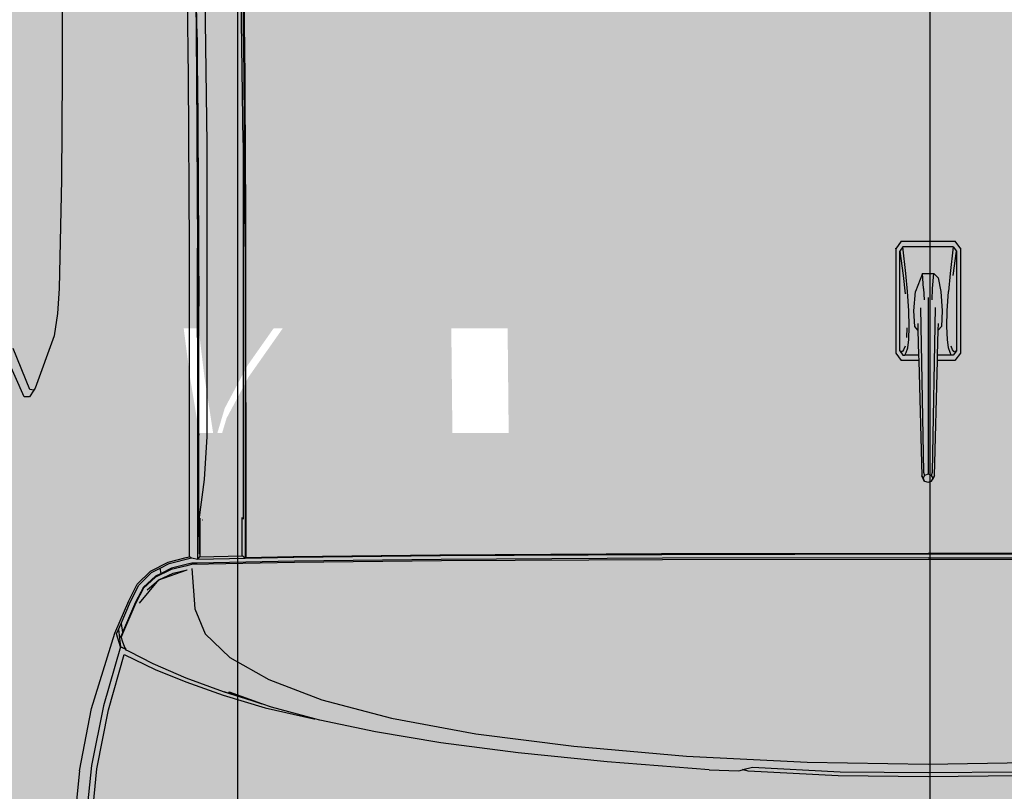
# Model space of a CAD drawing. Units: inches. Extents: x 1884 to 2398, y 474 to 1488.
# Tile 6 of 39: x 2203 to 2232, y 597 to 620. Entities that reach past the tile are written whole.
import ezdxf

# ---------------------------------------------------------------- set-up
doc = ezdxf.new("R2010")
doc.units = ezdxf.units.IN
doc.header["$MEASUREMENT"] = 0
doc.layers.get('0').update_dxf_attribs({"color": 250})
doc.layers.add('A-ANNO-DIMS', color=2, linetype='Continuous', lineweight=18)
doc.layers.add('C-VEHI', color=8, linetype='Continuous', lineweight=18)
doc.layers.add('Edges', color=250, linetype='Continuous')
doc.layers.add('L-PVMT-PATT', color=9, linetype='Continuous', lineweight=13, true_color=0xc7c8ca)
doc.styles.get("Standard").update_dxf_attribs({"font": 'arial.ttf'})
doc.dimstyles.get("Standard").update_dxf_attribs({"dimtxt": 7, "dimasz": 0.18, "dimexe": 0.18, "dimexo": 0.0625, "dimgap": 0.09, "dimtad": 0, "dimtih": 1, "dimtoh": 1, "dimzin": 0, "dimdsep": 46, "dimlunit": 3, "dimtxsty": 'Standard', "dimcen": 0.09, "dimadec": 0, "dimazin": 0, "dimtfac": 1, "dimtofl": 0, "dimtmove": 0, "dimatfit": 3, "dimfxl": 1, "dimtolj": 1, "dimtzin": 0, "dimarcsym": 0})

# ---------------------------------------------------------------- blocks, each defined once
blk = doc.blocks.new('Nissan Qashqai pl')
at = {"layer": 'Edges'}
for p, q in [((11.05474, 11.92208), (11.05507, 12.12031)), ((11.05537, 11.92208), (11.05571, 12.1202)), ((11.0586, 12.11975), (11.05827, 11.92208)), ((11.05972, 12.11965), (11.05938, 11.92208)), ((11.21164, 11.92208), (11.21014, 12.01197)), ((11.22044, 11.98904), (11.22108, 11.92208)), ((11.21801, 11.92208), (11.21745, 11.98742)), ((10.8228, 11.94208), (10.82834, 11.94608)), ((10.82794, 11.94608), (10.82834, 11.94608)), ((10.82834, 11.94608), (10.90603, 11.94608)), ((10.90603, 11.94608), (10.91157, 11.94208)), ((10.8228, 11.94208), (10.82239, 11.94208)), ((10.8228, 11.90208), (10.8228, 11.94208)), ((10.82696, 11.94083), (10.83007, 11.94308)), ((10.82696, 11.94083), (10.82696, 11.90333)), ((10.82696, 11.94083), (10.84666, 11.93861)), ((10.84833, 11.9406), (10.83007, 11.94308)), ((10.83007, 11.94308), (10.9043, 11.94308)), ((10.84666, 11.93861), (10.86027, 11.93735)), ((10.8746, 11.93634), (10.86027, 11.93735)), ((10.90215, 11.93722), (10.89593, 11.93645)), ((10.90348, 11.94026), (10.90076, 11.93914)), ((10.90565, 11.93837), (10.90215, 11.93722)), ((10.90503, 11.94137), (10.90348, 11.94026)), ((10.9043, 11.94308), (10.90741, 11.94083)), ((10.9043, 11.94308), (10.90503, 11.94137)), ((10.90744, 11.9393), (10.90565, 11.93837)), ((10.90741, 11.94083), (10.90744, 11.9393)), ((10.90744, 11.9393), (10.90744, 11.92915)), ((10.91157, 11.94208), (10.91157, 11.92904)), ((10.85007, 11.92947), (10.86027, 11.93157)), ((10.86027, 11.93157), (10.8746, 11.93265)), ((10.88611, 11.93611), (10.8746, 11.93634)), ((10.8746, 11.93265), (10.88611, 11.93193)), ((10.889, 11.92962), (10.88395, 11.92975)), ((10.89593, 11.93645), (10.88611, 11.93611)), ((10.88611, 11.93193), (10.889, 11.92962)), ((10.84666, 11.92634), (10.85007, 11.92947)), ((10.84666, 11.91782), (10.84666, 11.92634)), ((10.85787, 11.92547), (10.84666, 11.92634)), ((10.86624, 11.92503), (10.85787, 11.92547)), ((10.99456, 11.92544), (10.87195, 11.92764)), ((10.90744, 11.92915), (10.889, 11.92962)), ((10.91157, 11.92904), (10.90744, 11.92915)), ((10.99731, 11.92683), (10.91157, 11.92904)), ((10.99691, 11.92468), (10.99456, 11.92544)), ((10.99691, 11.92468), (10.99603, 11.92208)), ((10.99903, 11.92575), (10.99691, 11.92468)), ((10.99731, 11.92683), (11.00007, 11.92544)), ((10.99903, 11.92575), (10.99731, 11.92683)), ((11.00116, 11.92468), (10.99903, 11.92575)), ((11.00116, 11.92468), (11.00007, 11.92544)), ((11.00204, 11.92208), (11.00116, 11.92468)), ((10.85787, 11.91869), (10.84666, 11.91782)), ((10.84666, 11.91782), (10.86027, 11.91259)), ((10.85787, 11.91869), (10.86624, 11.91913)), ((10.86474, 11.92208), (10.99603, 11.92208)), ((10.87225, 11.91653), (10.99456, 11.91872)), ((10.90744, 11.91502), (10.91157, 11.91512)), ((10.91157, 11.91512), (10.99731, 11.91733)), ((10.91157, 11.91512), (10.91157, 11.90208)), ((10.99456, 11.91872), (10.99691, 11.91949)), ((10.99603, 11.92208), (10.99691, 11.91949)), ((10.99691, 11.91949), (10.99903, 11.91841)), ((11.00007, 11.91872), (10.99731, 11.91733)), ((10.99731, 11.91733), (10.99903, 11.91841)), ((10.99903, 11.91841), (10.99963, 11.91871)), ((10.99963, 11.91871), (11.00116, 11.91949)), ((11.00007, 11.91872), (10.99963, 11.91871)), ((11.00116, 11.91949), (11.00007, 11.91872)), ((11.00116, 11.91949), (11.00204, 11.92208)), ((11.05507, 11.72385), (11.05474, 11.92208)), ((11.05571, 11.72396), (11.05537, 11.92208)), ((11.05827, 11.92208), (11.0586, 11.72441)), ((11.05938, 11.92208), (11.05972, 11.72451)), ((11.21014, 11.8322), (11.21164, 11.92208)), ((11.21745, 11.85674), (11.21801, 11.92208)), ((11.22108, 11.92208), (11.22044, 11.85512)), ((10.8746, 11.91151), (10.86027, 11.91259)), ((10.8746, 11.90782), (10.86027, 11.90681)), ((10.88611, 11.91223), (10.8746, 11.91151)), ((10.88611, 11.90805), (10.8746, 11.90782)), ((10.88395, 11.91441), (10.889, 11.91454)), ((10.889, 11.91454), (10.88611, 11.91223)), ((10.89593, 11.90771), (10.88611, 11.90805)), ((10.889, 11.91454), (10.90744, 11.91502)), ((10.90744, 11.91502), (10.90744, 11.90486)), ((10.82239, 11.90208), (10.8228, 11.90208)), ((10.8228, 11.90208), (10.82834, 11.89808)), ((10.84666, 11.90555), (10.82696, 11.90333)), ((10.82696, 11.90333), (10.83007, 11.90108)), ((10.83007, 11.90108), (10.84833, 11.90356)), ((10.9043, 11.90108), (10.83007, 11.90108)), ((10.86027, 11.90681), (10.84666, 11.90555)), ((10.84833, 11.90356), (10.86193, 11.905)), ((10.88709, 11.90634), (10.89442, 11.90601)), ((10.90215, 11.90694), (10.89593, 11.90771)), ((10.90076, 11.90502), (10.90348, 11.9039)), ((10.90565, 11.90579), (10.90215, 11.90694)), ((10.90348, 11.9039), (10.90503, 11.90279)), ((10.9043, 11.90108), (10.90741, 11.90333)), ((10.90503, 11.90279), (10.9043, 11.90108)), ((10.90744, 11.90486), (10.90565, 11.90579)), ((10.90603, 11.89808), (10.91157, 11.90208)), ((10.90741, 11.90333), (10.90744, 11.90486)), ((10.90741, 11.90333), (10.90741, 11.90484)), ((10.82834, 11.89808), (10.82794, 11.89808)), ((10.82834, 11.89808), (10.90603, 11.89808)), ((11.2139, 11.7914), (11.21745, 11.85674)), ((11.22044, 11.85512), (11.21682, 11.78816)), ((11.20565, 11.74231), (11.21014, 11.8322)), ((11.21579, 11.78424), (11.2139, 11.7914)), ((11.21682, 11.78816), (11.21579, 11.78424)), ((11.21585, 11.78401), (11.21579, 11.78424)), ((11.21682, 11.78816), (11.21585, 11.78401)), ((11.21658, 11.78121), (11.21585, 11.78401)), ((11.21586, 11.75915), (11.21658, 11.78121)), ((11.21586, 11.75915), (11.20997, 11.68347)), ((11.19842, 11.65867), (11.20565, 11.74231)), ((11.05596, 11.55904), (11.05507, 11.72385)), ((11.0566, 11.5593), (11.05571, 11.72396)), ((11.0586, 11.72441), (11.05947, 11.55994)), ((11.05972, 11.72451), (11.06059, 11.56009)), ((11.20997, 11.68347), (11.2033, 11.61723)), ((11.18907, 11.58559), (11.19842, 11.65867)), ((11.2033, 11.61723), (11.19582, 11.55976)), ((11.17758, 11.52307), (11.18907, 11.58559)), ((11.05722, 11.44991), (11.05596, 11.55904)), ((11.05785, 11.45038), (11.0566, 11.5593)), ((11.05947, 11.55994), (11.06074, 11.45082)), ((11.06059, 11.56009), (11.06182, 11.4509)), ((11.19582, 11.55976), (11.18773, 11.51111)), ((11.16395, 11.47112), (11.17758, 11.52307)), ((11.18773, 11.51111), (11.17906, 11.46956)), ((11.14869, 11.43161), (11.16395, 11.47112)), ((11.17906, 11.46956), (11.17808, 11.46592)), ((11.17808, 11.46592), (11.1694, 11.43374)), ((11.1699, 11.42889), (11.17797, 11.4652)), ((11.17797, 11.4652), (11.17808, 11.46592)), ((11.05789, 11.4146), (11.05722, 11.44991)), ((11.05854, 11.41419), (11.05785, 11.45038)), ((11.06074, 11.45082), (11.06214, 11.37845)), ((11.06182, 11.4509), (11.06324, 11.37414)), ((11.1694, 11.43374), (11.1668, 11.42651)), ((11.1323, 11.40268), (11.14869, 11.43161)), ((11.1668, 11.42651), (11.1582, 11.40259)), ((11.16047, 11.39766), (11.1699, 11.42889)), ((11.16426, 11.41918), (11.1668, 11.42651)), ((11.15764, 11.39828), (11.16426, 11.41918)), ((11.15766, 11.39771), (11.16426, 11.41918)), ((11.16426, 11.41918), (11.15826, 11.40186)), ((10.69961, 11.41337), (10.55607, 11.41187)), ((10.5563, 11.41232), (10.69989, 11.41381)), ((10.7493, 11.41253), (10.62233, 11.41086)), ((10.77221, 11.41378), (10.69961, 11.41337)), ((10.69989, 11.41381), (10.77221, 11.4142)), ((10.7493, 11.41253), (11.02943, 11.41262)), ((10.77221, 11.4142), (10.78885, 11.41429)), ((10.77221, 11.4142), (10.77221, 11.41378)), ((10.78885, 11.41387), (10.77221, 11.41378)), ((10.78885, 11.41429), (10.79225, 11.41431)), ((10.78885, 11.41387), (10.78885, 11.41429)), ((10.79225, 11.41389), (10.78885, 11.41387)), ((10.79225, 11.41431), (10.79328, 11.41432)), ((10.79225, 11.41389), (10.79225, 11.41431)), ((10.79328, 11.4139), (10.79225, 11.41389)), ((10.79328, 11.41432), (10.82704, 11.4145)), ((10.79328, 11.4139), (10.79328, 11.41432)), ((10.82673, 11.41408), (10.79328, 11.4139)), ((10.82673, 11.41408), (11.05854, 11.41419)), ((10.82704, 11.4145), (11.05789, 11.4146)), ((11.02945, 11.41183), (11.02814, 11.41183)), ((11.02944, 11.41252), (11.02943, 11.41262)), ((11.05683, 11.41184), (11.02945, 11.41183)), ((11.02945, 11.41162), (11.02945, 11.41183)), ((11.05854, 11.41419), (11.05683, 11.41184)), ((11.05743, 11.38044), (11.05683, 11.41184)), ((11.05854, 11.41419), (11.05789, 11.4146)), ((11.05921, 11.37886), (11.05854, 11.41419)), ((11.11477, 11.38434), (11.1323, 11.40268)), ((11.14751, 11.37001), (11.15766, 11.39771)), ((11.15051, 11.36998), (11.16047, 11.39766)), ((10.62366, 11.38388), (10.75022, 11.38554)), ((10.75022, 11.38554), (10.96805, 11.38566)), ((10.96805, 11.38566), (10.99996, 11.38365)), ((10.99996, 11.38365), (11.03007, 11.37965)), ((11.03002, 11.38217), (11.03001, 11.38239)), ((11.03005, 11.38043), (11.05544, 11.38044)), ((11.05544, 11.38044), (11.03005, 11.38025)), ((11.05544, 11.38044), (11.05743, 11.38044)), ((11.05921, 11.37886), (11.05743, 11.38044)), ((11.09618, 11.37663), (11.11477, 11.38434)), ((10.55662, 11.37645), (10.69998, 11.37799)), ((10.6649, 11.37825), (10.55757, 11.37665)), ((10.6649, 11.37825), (10.58658, 11.37719)), ((10.69078, 11.37855), (10.6649, 11.37825)), ((10.6649, 11.37825), (10.67717, 11.37844)), ((10.69658, 11.37873), (10.67717, 11.37844)), ((10.67717, 11.37844), (10.69078, 11.37855)), ((10.69913, 11.37864), (10.69078, 11.37855)), ((10.71439, 11.37882), (10.69658, 11.37873)), ((10.69986, 11.37862), (10.69913, 11.37864)), ((10.69986, 11.37862), (10.78083, 11.37927)), ((10.71439, 11.37882), (10.69986, 11.37862)), ((10.69998, 11.37799), (10.82786, 11.37874)), ((10.72388, 11.37887), (10.71439, 11.37882)), ((10.72479, 11.37891), (10.72388, 11.37887)), ((10.78083, 11.37927), (10.72479, 11.37891)), ((10.78083, 11.37927), (10.8711, 11.37956)), ((10.94306, 11.3796), (10.82786, 11.37874)), ((10.82786, 11.37874), (11.05524, 11.37886)), ((10.96142, 11.37881), (10.82786, 11.37874)), ((10.89604, 11.37957), (10.8711, 11.37956)), ((10.90974, 11.3796), (10.89604, 11.37957)), ((10.94306, 11.3796), (10.90974, 11.3796)), ((10.94785, 11.37963), (10.94306, 11.3796)), ((10.9491, 11.37964), (10.94785, 11.37963)), ((10.96679, 11.37961), (10.9491, 11.37964)), ((10.96142, 11.37881), (10.96679, 11.37961)), ((10.97113, 11.37881), (10.96142, 11.37881)), ((10.96679, 11.37961), (10.96696, 11.37964)), ((10.97653, 11.37962), (10.96696, 11.37964)), ((10.97653, 11.37962), (10.97113, 11.37881)), ((10.97664, 11.37882), (10.97113, 11.37881)), ((10.98248, 11.37964), (10.97653, 11.37962)), ((10.97653, 11.37962), (10.97664, 11.37882)), ((11.05921, 11.37886), (10.97664, 11.37882)), ((11.03007, 11.37965), (10.98248, 11.37964)), ((11.02869, 11.38043), (11.03005, 11.38043)), ((11.03005, 11.38025), (11.02923, 11.38024)), ((11.03005, 11.38025), (11.03005, 11.38043)), ((11.03007, 11.37965), (11.03005, 11.38025)), ((11.05822, 11.37418), (11.05754, 11.37277)), ((11.05822, 11.37418), (11.05921, 11.37886)), ((11.06236, 11.3576), (11.05822, 11.37418)), ((11.06214, 11.37845), (11.06222, 11.37449)), ((11.06222, 11.37449), (11.06303, 11.37135)), ((11.06324, 11.37414), (11.06408, 11.37085)), ((11.06624, 11.37435), (11.09618, 11.37663)), ((10.7004, 11.37196), (10.55723, 11.37045)), ((10.82794, 11.37265), (10.7004, 11.37196)), ((11.05437, 11.37279), (10.82794, 11.37265)), ((11.05754, 11.37277), (11.05437, 11.37279)), ((11.05807, 11.37037), (11.05754, 11.37277)), ((11.06139, 11.35691), (11.05807, 11.37037)), ((11.06303, 11.37135), (11.06594, 11.3594)), ((11.06408, 11.37085), (11.06692, 11.35921)), ((11.06961, 11.36056), (11.0671, 11.37109)), ((11.07472, 11.34981), (11.0671, 11.37109)), ((11.13692, 11.34555), (11.14751, 11.37001)), ((11.14123, 11.34726), (11.15051, 11.36998)), ((11.06594, 11.3594), (11.06978, 11.35164)), ((11.06692, 11.35921), (11.0727, 11.34754)), ((11.07472, 11.34981), (11.06961, 11.36056)), ((11.06818, 11.34377), (11.06139, 11.35691)), ((11.06584, 11.35092), (11.06236, 11.3576)), ((11.06978, 11.35164), (11.06584, 11.35092)), ((11.06978, 11.35164), (11.07183, 11.3475)), ((11.06918, 11.34452), (11.06584, 11.35092)), ((11.07866, 11.33492), (11.06918, 11.34452)), ((11.07183, 11.3475), (11.08018, 11.33842)), ((11.0727, 11.34754), (11.0809, 11.33858)), ((11.08206, 11.34125), (11.07472, 11.34981)), ((11.092, 11.33548), (11.07472, 11.34981)), ((11.12767, 11.32749), (11.13692, 11.34555)), ((11.13017, 11.32416), (11.14123, 11.34726)), ((11.07787, 11.3339), (11.06818, 11.34377)), ((11.08018, 11.33842), (11.09121, 11.33249)), ((11.0809, 11.33858), (11.09174, 11.33271)), ((11.09022, 11.32753), (11.07787, 11.3339)), ((11.09081, 11.32882), (11.07866, 11.33492)), ((11.09121, 11.33249), (11.1138, 11.3229)), ((11.09174, 11.33271), (11.11486, 11.323)), ((11.11439, 11.31711), (11.09022, 11.32753)), ((11.10704, 11.32181), (11.09081, 11.32882)), ((11.10704, 11.32181), (11.1138, 11.3229)), ((11.1138, 11.3229), (11.11393, 11.32284)), ((11.11393, 11.32284), (11.1164, 11.32172)), ((11.11486, 11.323), (11.1172, 11.32196)), ((11.1164, 11.32172), (11.1172, 11.32196)), ((11.11744, 11.32189), (11.1164, 11.32172)), ((11.1172, 11.32196), (11.11744, 11.32189)), ((11.11744, 11.32189), (11.11997, 11.32267)), ((11.11997, 11.32267), (11.12459, 11.32429)), ((11.12604, 11.32481), (11.1244, 11.32146)), ((11.1244, 11.32146), (11.12591, 11.32476)), ((11.12459, 11.32429), (11.12591, 11.32476)), ((11.12466, 11.32442), (11.12595, 11.32486)), ((11.12478, 11.32467), (11.12595, 11.32486)), ((11.12595, 11.32486), (11.1251, 11.3253)), ((11.12591, 11.32476), (11.12595, 11.32486)), ((11.12591, 11.32476), (11.12604, 11.32481)), ((11.12595, 11.32486), (11.12626, 11.32554)), ((11.12595, 11.32486), (11.12607, 11.32488)), ((11.12604, 11.32481), (11.12645, 11.32495)), ((11.12607, 11.32488), (11.12604, 11.32481)), ((11.12631, 11.32537), (11.12607, 11.32488)), ((11.12607, 11.32488), (11.12645, 11.32495)), ((11.12645, 11.32495), (11.12767, 11.32749)), ((11.17121, 11.31245), (11.13017, 11.32416)), ((11.11164, 11.31982), (11.10704, 11.32181)), ((11.11164, 11.31982), (11.1244, 11.32146)), ((11.11467, 11.31851), (11.11164, 11.31982)), ((11.17021, 11.29978), (11.11439, 11.31711)), ((11.1244, 11.32146), (11.11467, 11.31851)), ((11.1244, 11.32146), (11.16836, 11.30873)), ((11.16836, 11.30873), (11.21271, 11.29983)), ((11.21523, 11.3038), (11.17121, 11.31245)), ((11.2509, 11.3003), (11.21523, 11.3038)), ((11.21656, 11.2908), (11.17021, 11.29978)), ((11.21271, 11.29983), (11.24875, 11.29618)), ((11.21656, 11.2908), (11.25377, 11.28706)), ((10.58925, 11.27827), (10.69879, 11.27793)), ((10.69879, 11.27793), (10.77686, 11.27742)), ((10.77686, 11.27742), (10.85804, 11.27587)), ((10.85804, 11.27587), (10.87661, 11.27449)), ((10.87661, 11.27449), (10.89318, 11.27219)), ((10.89318, 11.27219), (10.932, 11.25799)), ((10.932, 11.25799), (10.93345, 11.25704)), ((10.93345, 11.25704), (10.93299, 11.25409)), ((10.93345, 11.25704), (10.93862, 11.25365)), ((10.93299, 11.25409), (10.90264, 11.24169)), ((10.9384, 11.24966), (10.90591, 11.23547)), ((10.93862, 11.25365), (10.9384, 11.24966))]:
    blk.add_line(p, q, dxfattribs=at)
blk = doc.blocks.new('car')
blk.add_blockref('Nissan Qashqai pl', (-9.74328, -11.91512))
blk = doc.blocks.new('carr')
blk.add_blockref('car', (0.51244, -0.00696))
blk = doc.blocks.new('*D44')
at = {"layer": 'A-ANNO-DIMS', "color": 0, "lineweight": -2, "transparency": 16777216}
for p, q in [((2209.755, 1247.822), (2209.755, 484.005)), ((2230.029, 1247.822), (2230.029, 484.005)), ((2209.935, 484.185), (2229.849, 484.185)), ((2230.029, 484.185), (2230.209, 484.185))]:
    blk.add_line(p, q, dxfattribs=at)
at = {"layer": 'A-ANNO-DIMS', "color": 0, "lineweight": 100, "transparency": 16777216}
for points in [[(2209.935, 484.215), (2209.935, 484.155), (2209.755, 484.185)], [(2229.849, 484.215), (2229.849, 484.155), (2230.029, 484.185)]]:
    blk.add_solid(points, dxfattribs=at)
at = {"layer": 'Defpoints', "color": 0, "lineweight": 100, "transparency": 16777216}
for p in [(2209.755, 1247.885), (2230.029, 1247.885), (2230.029, 484.185)]:
    blk.add_point(p, dxfattribs=at)
at = {"layer": 'A-ANNO-DIMS', "color": 0, "transparency": 16777216, "insert": (2247.429, 484.185), "char_height": 7, "attachment_point": 5}
blk.add_mtext('\\A1;1\'-8 1/2"', dxfattribs=at)

msp = doc.modelspace()

# ---------------------------------------------------------------- hatches: boundary and pattern name
at = {"layer": 'L-PVMT-PATT'}
h = msp.add_hatch(color=256, dxfattribs=at)
h.dxf.hatch_style = 1
h.paths.add_polyline_path([(2387.529, 769.966), (2351.529, 769.966), (2238.447, 769.966), (2238.447, 762.15), (2238.447, 754.445), (2126.529, 754.445), (2126.529, 676.183), (2134.868, 676.183), (2142.673, 676.183), (2142.673, 646.578), (2134.868, 646.578), (2126.529, 646.578), (2126.529, 640.17), (2387.529, 640.17)])
h.paths.add_polyline_path([(2387.529, 631.385), (2303.086, 631.385), (2303.086, 615.671), (2387.529, 615.671)])
h.paths.add_polyline_path([(2387.529, 640.17), (2126.529, 640.17), (2126.529, 631.385), (2387.529, 631.385)])
h.paths.add_polyline_path([(2393.529, 604.13), (2387.529, 604.13), (2387.529, 615.671), (2303.086, 615.671), (2303.086, 607.943), (2249.649, 607.943), (2126.529, 607.943), (2126.529, 533.885), (2393.529, 533.885)])
h.paths.add_polyline_path([(2257.825, 611.008), (2257.83, 611.337), (2257.915, 616.493), (2258.021, 621.805), (2258.146, 627.274), (2258.252, 631.385), (2126.529, 631.385), (2126.529, 611.008)])
h.paths.add_polyline_path([(2258.892, 611.285), (2258.888, 611.008), (2300.247, 611.008), (2300.247, 631.385), (2259.314, 631.385), (2259.206, 627.173), (2259.081, 621.72), (2258.976, 616.424)])
h = msp.add_hatch(color=256, dxfattribs=at)
h.dxf.hatch_style = 1
h.paths.add_polyline_path([(2216.015, 611.008), (2212.351, 611.008), (2212.342, 608.327), (2212.34, 607.943), (2216.046, 607.943), (2216.044, 608.264)])
h.paths.add_polyline_path([(2212.351, 611.008), (2211.081, 611.008), (2210.074, 609.575), (2209.435, 608.376), (2209.305, 607.943), (2212.34, 607.943), (2212.342, 608.327)])
h.paths.add_polyline_path([(2257.742, 611.008), (2249.649, 611.008), (2217.664, 611.008), (2217.692, 608.284), (2217.694, 607.943), (2249.649, 607.943), (2257.712, 607.943), (2257.713, 608.284)])
h.paths.add_polyline_path([(2266.79, 611.008), (2264.592, 611.008), (2265.355, 609.923), (2266.022, 608.672), (2266.241, 607.943), (2266.364, 607.943), (2266.622, 609.602)])
h.paths.add_polyline_path([(2263.055, 611.008), (2259.39, 611.008), (2259.361, 608.264), (2259.359, 607.943), (2263.065, 607.943), (2263.063, 608.327)])
h.paths.add_polyline_path([(2265.331, 609.575), (2264.325, 611.008), (2263.055, 611.008), (2263.063, 608.327), (2263.065, 607.943), (2266.1, 607.943), (2265.97, 608.376)])
h.paths.add_polyline_path([(2272.885, 609.347), (2272.901, 609.457), (2272.902, 609.679), (2272.895, 611.008), (2271.456, 611.008), (2271.351, 610.147), (2271.277, 610.077), (2270.912, 610.081), (2270.481, 610.11), (2270.455, 610.183), (2270.448, 611.008), (2269.23, 611.008), (2269.228, 610.963), (2269.055, 608.458), (2269.014, 607.943), (2272.869, 607.943), (2272.882, 607.958)])
h.paths.add_polyline_path([(2269.228, 610.963), (2269.23, 611.008), (2267.227, 611.008), (2267.038, 609.547), (2266.77, 607.943), (2269.014, 607.943), (2269.055, 608.458)])
h.paths.add_polyline_path([(2293.178, 611.008), (2272.917, 611.008), (2272.925, 609.643), (2272.924, 609.184), (2272.925, 609.03), (2272.921, 607.943), (2293.123, 607.943), (2293.127, 608.565), (2293.159, 610.362)])
h.paths.add_polyline_path([(2302.932, 613.651), (2302.931, 615.98), (2302.91, 623.22), (2302.851, 630.905), (2302.844, 631.385), (2300.247, 631.385), (2300.247, 612.163), (2300.885, 611.925), (2301.121, 611.86), (2301.743, 612.576)])
h.paths.add_polyline_path([(2302.992, 610.861), (2302.993, 612.796), (2302.965, 612.8), (2301.576, 611.546), (2300.954, 610.83), (2300.899, 610.766), (2300.444, 610.894), (2300.139, 611.008), (2299.369, 611.008), (2299.448, 609.776), (2299.311, 611.008), (2299.207, 611.008), (2299.34, 609.722), (2299.553, 607.943), (2300.825, 607.943), (2300.851, 607.993), (2301.87, 609.442)])
h.paths.add_polyline_path([(2298.512, 611.008), (2296.882, 611.008), (2296.979, 609.034), (2297.054, 607.943), (2298.828, 607.943), (2298.736, 608.659)])
h.paths.add_polyline_path([(2294.51, 608.662), (2294.51, 608.662), (2294.362, 610.672), (2294.359, 611.008), (2293.338, 611.008), (2293.331, 610.606), (2293.329, 610.538), (2293.315, 609.691), (2293.305, 607.943), (2294.597, 607.943)])
h.paths.add_polyline_path([(2302.991, 609.68), (2301.718, 608.051), (2301.642, 607.943), (2302.986, 607.943)], flags=17)
h = msp.add_hatch(color=256, dxfattribs=at)
h.dxf.hatch_style = 1
h.paths.add_polyline_path([(2202.48, 609.653), (2202.489, 611.008), (2126.529, 611.008), (2126.529, 607.943), (2202.484, 607.943), (2202.48, 609.055), (2202.481, 609.184)])
h.paths.add_polyline_path([(2210.813, 611.008), (2208.615, 611.008), (2208.784, 609.602), (2209.041, 607.943), (2209.165, 607.943), (2209.383, 608.672), (2210.05, 609.923)])
h.paths.add_polyline_path([(2208.179, 611.008), (2206.175, 611.008), (2206.177, 610.963), (2206.351, 608.458), (2206.392, 607.943), (2208.635, 607.943), (2208.367, 609.547)])
h.paths.add_polyline_path([(2206.177, 610.963), (2206.175, 611.008), (2204.958, 611.008), (2204.951, 610.183), (2204.925, 610.11), (2204.493, 610.081), (2204.129, 610.077), (2204.054, 610.147), (2203.949, 611.008), (2202.51, 611.008), (2202.503, 609.679), (2202.511, 607.972), (2202.537, 607.943), (2206.392, 607.943), (2206.351, 608.458)])
h.paths.add_polyline_path([(2204.425, 611.008), (2203.949, 611.008), (2204.054, 610.147), (2204.489, 610.176)], flags=17)
h.paths.add_polyline_path([(2204.958, 611.008), (2204.517, 611.008), (2204.581, 610.179), (2204.951, 610.183)], flags=17)
h.paths.add_polyline_path([(2204.517, 611.008), (2204.425, 611.008), (2204.489, 610.176), (2204.581, 610.179)], flags=17)
h.paths.add_polyline_path([(2204.489, 610.176), (2204.054, 610.147), (2204.129, 610.077), (2204.485, 610.101), (2204.561, 610.106)], flags=17)
h.paths.add_polyline_path([(2204.581, 610.179), (2204.489, 610.176), (2204.561, 610.106)], flags=17)
h.paths.add_polyline_path([(2204.951, 610.183), (2204.581, 610.179), (2204.561, 610.106), (2204.925, 610.11)], flags=17)
h.paths.add_polyline_path([(2204.925, 610.11), (2204.561, 610.106), (2204.485, 610.101), (2204.493, 610.081)], flags=17)
h.paths.add_polyline_path([(2204.485, 610.101), (2204.129, 610.077), (2204.493, 610.081)], flags=16)

# ---------------------------------------------------------------- block references
at = {"layer": 'C-VEHI', "xscale": 39.37007874015748, "yscale": 39.37007874015748, "zscale": 39.37007874015748, "rotation": 270}
msp.add_blockref('carr', (2229.977, 676.232), dxfattribs=at)

# ---------------------------------------------------------------- dimensions: what is measured, and where the dimension line sits
at = {"layer": 'A-ANNO-DIMS'}
dim = msp.add_linear_dim(base=(2230.029, 484.185), p1=(2209.755, 1247.885), p2=(2230.029, 1247.885), dimstyle='Standard', override={"dimdec": 1, "dimlfac": 1, "dimrnd": 0, "dimzin": 1, "dimdsep": 46, "dimlunit": 4, "dimfrac": 2}, dxfattribs=at)
dim.commit()
dim.dimension.update_dxf_attribs({"geometry": '*D44', "text_midpoint": (2247.429, 484.185)})

doc.saveas('drawing.dxf')
